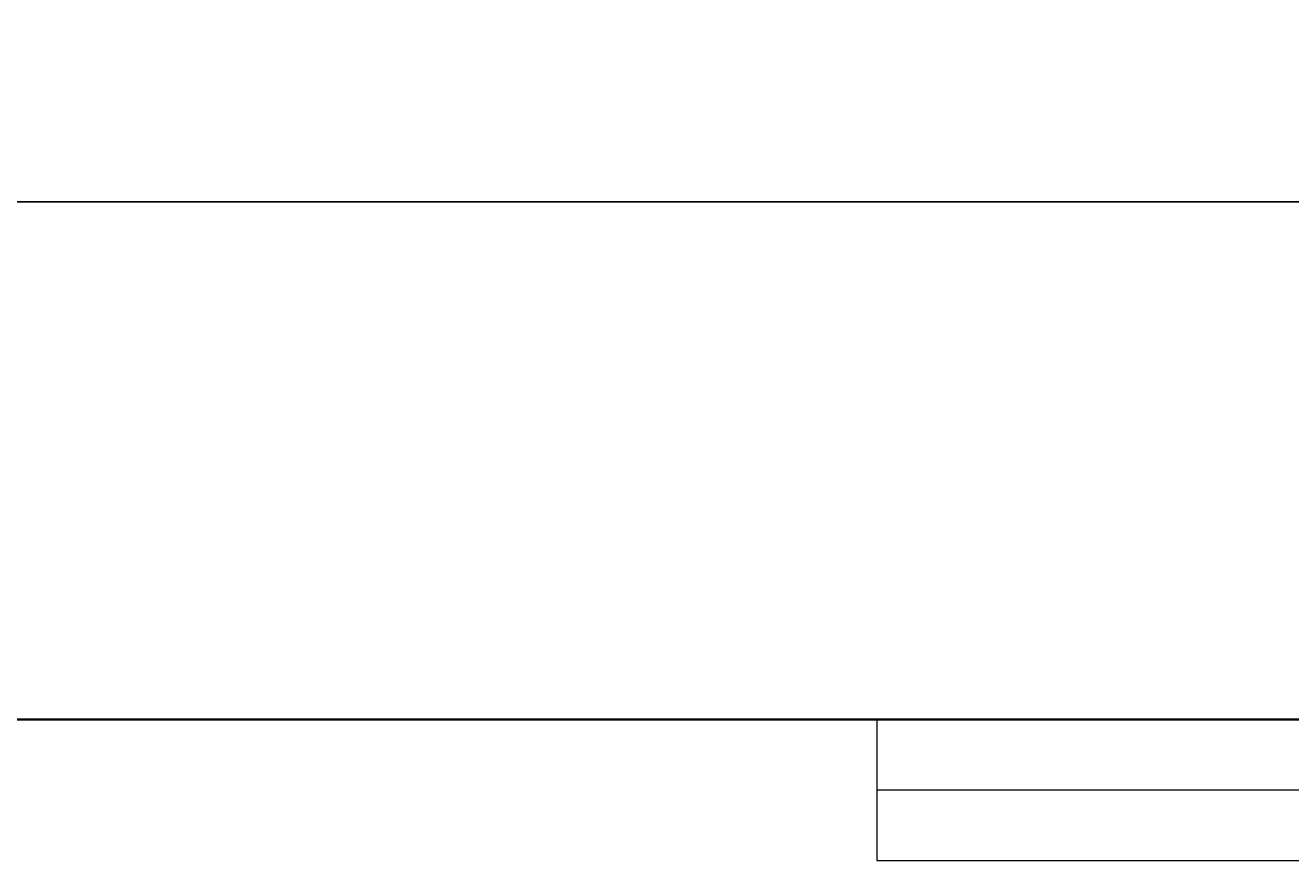
# Model space of a CAD drawing. Units: millimetres. Extents: x 27017497 to 27018854, y 7058029 to 7059154.
# Tile 87 of 91: x 27018319 to 27018399, y 7058581 to 7058634. Entities that reach past the tile are written whole.
import ezdxf

# ---------------------------------------------------------------- set-up
doc = ezdxf.new("R2010")
doc.units = ezdxf.units.MM
for name, color, linetype, lineweight in [('A-ANNO-DIMS', 2, 'Continuous', 18), ('A-GLAZ', 4, 'Continuous', 18), ('A-WALL', 7, 'Continuous', 35)]:
    doc.layers.add(name, color=color, linetype=linetype, lineweight=lineweight)
doc.styles.get("Standard").update_dxf_attribs({"font": 'arial.ttf'})
doc.dimstyles.get("Standard").update_dxf_attribs({"dimtxt": 0.18, "dimasz": 0.18, "dimexe": 0.18, "dimexo": 0.0625, "dimgap": 0.09, "dimtad": 0, "dimtih": 1, "dimtoh": 1, "dimdec": 4, "dimzin": 0, "dimdsep": 46, "dimtxsty": 'Standard', "dimcen": 0.09, "dimadec": 0, "dimazin": 0, "dimtfac": 1, "dimtdec": 4, "dimtofl": 0, "dimtmove": 0, "dimatfit": 3, "dimfxl": 1, "dimtolj": 1, "dimtzin": 0, "dimarcsym": 0})

# ---------------------------------------------------------------- blocks, each defined once
blk = doc.blocks.new('WINDOW-SINGLE-LIGHT')
blk.add_lwpolyline([(36, 4.5), (36, 0), (0, 0), (0, 9), (36, 9), (36, 4.5), (0, 4.5)])
blk = doc.blocks.new('*D48')
at = {"layer": 'A-ANNO-DIMS', "color": 0, "lineweight": -2, "transparency": 16777216}
for p, q in [((27018463.498, 7058622.912), (27017497.536, 7058622.912)), ((27017497.716, 7058622.732), (27017497.716, 7058357.753)), ((27017497.716, 7058092.41), (27017497.716, 7058357.389)), ((27018555.129, 7058092.23), (27017497.536, 7058092.23))]:
    blk.add_line(p, q, dxfattribs=at)
at = {"layer": 'A-ANNO-DIMS', "color": 0, "transparency": 16777216}
for points in [[(27017497.686, 7058622.732), (27017497.746, 7058622.732), (27017497.716, 7058622.912)], [(27017497.686, 7058092.41), (27017497.746, 7058092.41), (27017497.716, 7058092.23)]]:
    blk.add_solid(points, dxfattribs=at)
at = {"layer": 'Defpoints', "color": 0, "transparency": 16777216}
for p in [(27018463.561, 7058622.912), (27017497.716, 7058092.23), (27018555.192, 7058092.23)]:
    blk.add_point(p, dxfattribs=at)
at = {"layer": 'A-ANNO-DIMS', "color": 0, "transparency": 16777216, "insert": (27017497.716, 7058357.571), "char_height": 0.18, "attachment_point": 5}
blk.add_mtext('\\A1;530.7', dxfattribs=at)
blk = doc.blocks.new('*D52')
at = {"layer": 'A-ANNO-DIMS', "color": 0, "lineweight": -2, "transparency": 16777216}
for p, q in [((27018310.606, 7058589.975), (27018310.606, 7058686.542)), ((27018310.786, 7058686.362), (27018523.958, 7058686.362)), ((27018737.926, 7058686.362), (27018524.754, 7058686.362)), ((27018738.106, 7058589.975), (27018738.106, 7058686.542))]:
    blk.add_line(p, q, dxfattribs=at)
at = {"layer": 'A-ANNO-DIMS', "color": 0, "transparency": 16777216}
for points in [[(27018310.786, 7058686.392), (27018310.786, 7058686.332), (27018310.606, 7058686.362)], [(27018737.926, 7058686.392), (27018737.926, 7058686.332), (27018738.106, 7058686.362)]]:
    blk.add_solid(points, dxfattribs=at)
at = {"layer": 'Defpoints', "color": 0, "transparency": 16777216}
for p in [(27018738.106, 7058686.362), (27018310.606, 7058589.912), (27018738.106, 7058589.912)]:
    blk.add_point(p, dxfattribs=at)
at = {"layer": 'A-ANNO-DIMS', "color": 0, "transparency": 16777216, "insert": (27018524.356, 7058686.362), "char_height": 0.18, "attachment_point": 5}
blk.add_mtext('\\A1;427.5', dxfattribs=at)

msp = doc.modelspace()

# ---------------------------------------------------------------- linework, layer by layer
at = {"layer": 'A-WALL'}
msp.add_line((27018738.106, 7058589.912), (27018310.606, 7058589.912), dxfattribs=at)

# ---------------------------------------------------------------- block references
at = {"layer": 'A-GLAZ', "extrusion": (0, 0, -1), "zscale": -1}
msp.add_blockref('WINDOW-SINGLE-LIGHT', (-27018409.137, 7058580.929), dxfattribs=at)

# ---------------------------------------------------------------- dimensions: what is measured, and where the dimension line sits
at = {"layer": 'A-ANNO-DIMS'}
dim = msp.add_linear_dim(base=(27018738.106, 7058686.362), p1=(27018310.606, 7058589.912), p2=(27018738.106, 7058589.912), dimstyle='Standard', override={"dimdec": 1, "dimlfac": 1, "dimrnd": 0, "dimzin": 0, "dimdsep": 46, "dimlunit": 2}, dxfattribs=at)
dim.commit()
dim.dimension.update_dxf_attribs({"geometry": '*D52', "text_midpoint": (27018524.356, 7058686.362)})
dim = msp.add_linear_dim(base=(27017497.716, 7058092.23), p1=(27018463.561, 7058622.912), p2=(27018555.192, 7058092.23), angle=90, dimstyle='Standard', override={"dimdec": 1, "dimlfac": 1, "dimrnd": 0, "dimzin": 0, "dimdsep": 46, "dimlunit": 2}, dxfattribs=at)
dim.commit()
dim.dimension.update_dxf_attribs({"geometry": '*D48', "text_midpoint": (27017497.716, 7058357.571)})

doc.saveas('drawing.dxf')
